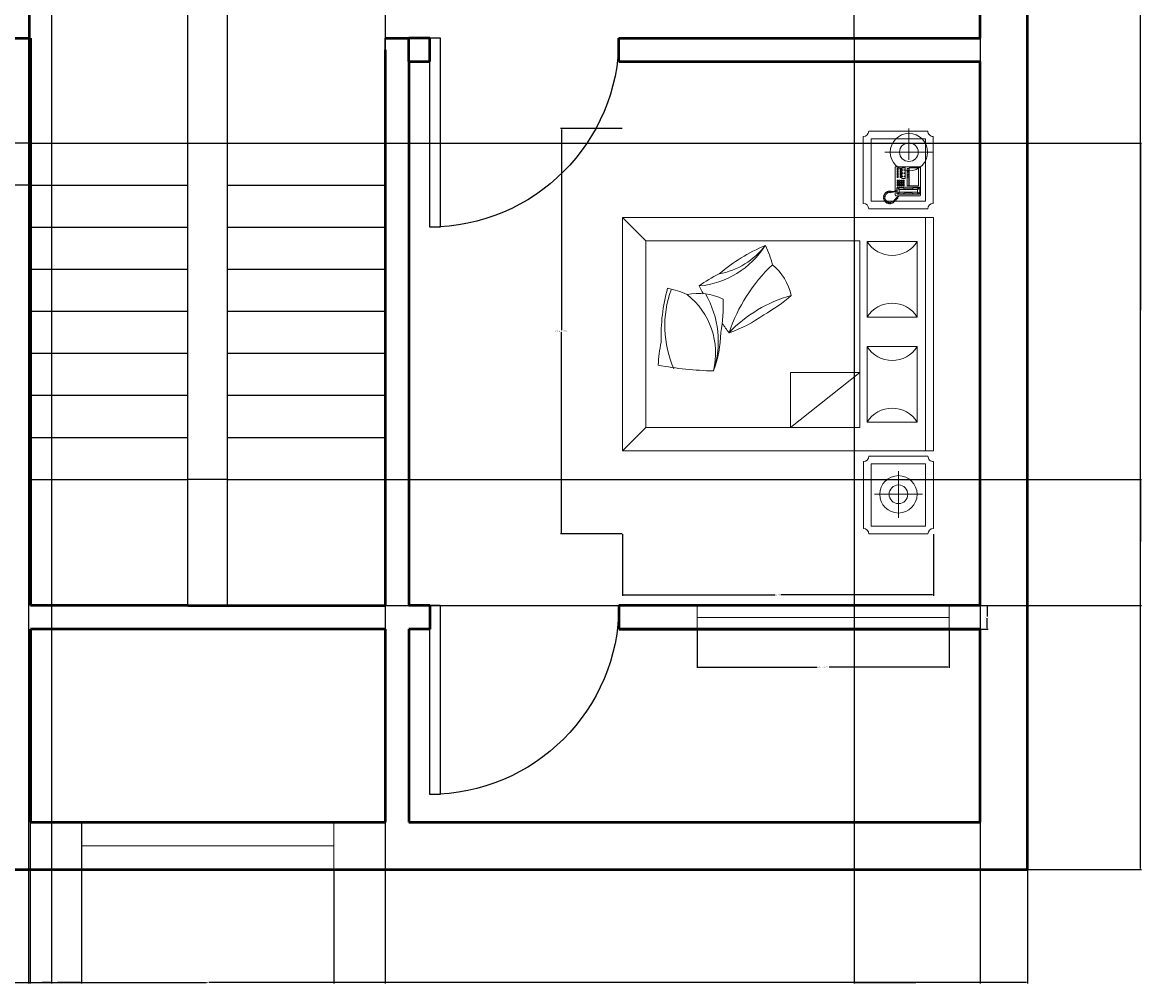
# Model space of a CAD drawing. Units: inches. Extents: x -108 to 1456, y -102 to 617.
# Tile 3 of 8: x 347 to 560, y 154 to 337. Entities that reach past the tile are written whole.
import ezdxf

# ---------------------------------------------------------------- set-up
doc = ezdxf.new("R2010")
doc.units = ezdxf.units.IN
for name, color, linetype, lineweight in [('A-ANNO-DIMS', 2, 'Continuous', 18), ('A-DOOR', 3, 'Continuous', 25), ('A-FLOR-CASE', 32, 'Continuous', 25), ('A-FLOR-STRS', 2, 'Continuous', 25), ('A-FURN', 8, 'Continuous', 18), ('A-GLAZ', 4, 'Continuous', 18), ('A-WALL', 7, 'Continuous', 50)]:
    doc.layers.add(name, color=color, linetype=linetype, lineweight=lineweight)
doc.styles.get("Standard").update_dxf_attribs({"font": 'arial.ttf'})
doc.dimstyles.get("Standard").update_dxf_attribs({"dimtxt": 0.18, "dimasz": 0.18, "dimexe": 0.18, "dimexo": 0.0625, "dimgap": 0.09, "dimtad": 0, "dimtih": 1, "dimtoh": 1, "dimdec": 4, "dimzin": 0, "dimdsep": 46, "dimtxsty": 'Standard', "dimcen": 0.09, "dimadec": 0, "dimazin": 0, "dimtfac": 1, "dimtdec": 4, "dimtofl": 0, "dimtmove": 0, "dimatfit": 3, "dimfxl": 1, "dimtolj": 1, "dimtzin": 0, "dimarcsym": 0})

# ---------------------------------------------------------------- blocks, each defined once
blk = doc.blocks.new('A$C50B66110')
for p, q in [((0.0153, 1.9631), (0.0153, 1.5831)), ((0.0503, 1.9981), (0.4803, 1.9981)), ((0.0653, 1.9481), (0.0653, 1.5981)), ((0.0653, 1.9481), (0.4653, 1.9481)), ((0.1513, 1.6871), (0.1513, 1.9967)), ((0.4653, 1.9481), (0.4653, 1.5981)), ((0.5153, 1.9631), (0.5153, 1.5831)), ((0.5716, 1.9488), (0.5716, 2)), ((0.5716, 2), (2.0719, 2)), ((2.0719, 1.9488), (0.5716, 1.9488)), ((0.5716, 1.9488), (0.5716, 0)), ((2.0719, 1.9488), (2.0719, 2)), ((2.0719, 0), (2.0719, 1.9488)), ((2.1051, 1.9643), (2.1051, 1.5843)), ((2.5701, 1.9993), (2.1401, 1.9993)), ((2.1551, 1.9493), (2.1551, 1.5993)), ((2.5551, 1.9493), (2.1551, 1.9493)), ((2.5551, 1.9493), (2.5551, 1.5993)), ((2.6051, 1.9643), (2.6051, 1.5843)), ((0.7257, 1.5725), (0.7257, 1.8954)), ((0.7257, 1.8954), (1.2113, 1.8954)), ((1.2113, 1.8954), (1.2113, 1.5725)), ((1.4007, 1.5725), (1.4007, 1.8954)), ((1.4007, 1.8954), (1.8863, 1.8954)), ((1.8863, 1.8954), (1.8863, 1.5725)), ((2.3505, 1.62), (2.3505, 1.9295)), ((0, 1.8416), (0.2001, 1.8416)), ((2.5018, 1.7744), (2.2017, 1.7744)), ((0.0653, 1.5981), (0.4653, 1.5981)), ((2.5551, 1.5993), (2.1551, 1.5993)), ((0.0503, 1.5481), (0.4803, 1.5481)), ((1.2113, 1.5725), (0.7257, 1.5725)), ((1.8863, 1.5725), (1.4007, 1.5725)), ((1.5665, 1.5254), (1.5665, 1.0802)), ((1.5665, 1.5254), (1.9219, 1.0802)), ((2.5701, 1.5493), (2.1401, 1.5493)), ((1.9219, 1.0802), (1.5665, 1.0802)), ((0.5716, 0), (0.7216, 0.15)), ((2.0719, 0), (1.9219, 0.15)), ((0.5716, 0), (2.0719, 0))]:
    blk.add_line(p, q)
at = {"linetype": 'ByBlock'}
for p, q in [((0.2481, 1.9162), (0.2458, 1.9139)), ((0.2458, 1.9139), (0.2458, 1.7562)), ((0.2481, 1.9162), (0.4287, 1.9162)), ((0.2526, 1.9036), (0.2526, 1.8431)), ((0.3669, 1.9036), (0.2526, 1.9036)), ((0.3669, 1.8431), (0.3669, 1.9036)), ((0.3772, 1.9071), (0.3818, 1.9128)), ((0.3772, 1.7688), (0.3772, 1.9071)), ((0.3818, 1.9094), (0.3807, 1.9048)), ((0.3807, 1.9048), (0.3807, 1.8739)), ((0.3807, 1.9048), (0.3909, 1.8945)), ((0.3807, 1.8739), (0.3829, 1.8682)), ((0.3818, 1.9128), (0.4161, 1.9128)), ((0.3864, 1.9116), (0.3818, 1.9094)), ((0.3921, 1.8968), (0.3864, 1.9116)), ((0.3864, 1.9116), (0.4138, 1.9116)), ((0.3909, 1.8945), (0.3921, 1.8968)), ((0.3909, 1.8431), (0.3909, 1.8945)), ((0.4081, 1.8968), (0.3921, 1.8968)), ((0.4081, 1.8968), (0.4138, 1.9116)), ((0.4092, 1.8945), (0.4081, 1.8968)), ((0.4195, 1.9048), (0.4092, 1.8945)), ((0.4092, 1.8431), (0.4092, 1.8945)), ((0.4138, 1.9116), (0.4184, 1.9094)), ((0.4161, 1.9128), (0.4218, 1.9071)), ((0.4195, 1.8739), (0.4172, 1.8682)), ((0.4184, 1.9094), (0.4195, 1.9048)), ((0.4195, 1.9048), (0.4195, 1.8739)), ((0.4218, 1.9071), (0.4218, 1.7699)), ((0.4287, 1.9162), (0.4309, 1.9139)), ((0.4309, 1.9139), (0.4309, 1.7562)), ((0.2526, 1.8431), (0.3669, 1.8431)), ((0.3201, 1.8168), (0.2526, 1.8168)), ((0.2526, 1.8168), (0.2526, 1.7962)), ((0.2572, 1.8408), (0.2572, 1.8294)), ((0.3669, 1.8408), (0.2572, 1.8408)), ((0.2572, 1.8294), (0.3669, 1.8294)), ((0.2675, 1.8145), (0.2641, 1.8145)), ((0.2641, 1.8145), (0.2641, 1.8111)), ((0.2641, 1.8111), (0.2675, 1.8111)), ((0.2641, 1.8019), (0.2641, 1.7985)), ((0.2675, 1.8019), (0.2641, 1.8019)), ((0.2641, 1.7985), (0.2675, 1.7985)), ((0.2664, 1.8408), (0.2664, 1.8294)), ((0.2675, 1.8111), (0.2675, 1.8145)), ((0.2675, 1.7985), (0.2675, 1.8019)), ((0.2755, 1.8408), (0.2755, 1.8294)), ((0.2846, 1.8408), (0.2846, 1.8294)), ((0.2846, 1.8145), (0.2846, 1.8111)), ((0.2881, 1.8145), (0.2846, 1.8145)), ((0.2846, 1.8111), (0.2881, 1.8111)), ((0.2846, 1.8019), (0.2846, 1.7985)), ((0.2881, 1.8019), (0.2846, 1.8019)), ((0.2846, 1.7985), (0.2881, 1.7985)), ((0.2881, 1.8111), (0.2881, 1.8145)), ((0.2881, 1.7985), (0.2881, 1.8019)), ((0.2938, 1.8408), (0.2938, 1.8294)), ((0.3029, 1.8408), (0.3029, 1.8294)), ((0.3052, 1.8145), (0.3052, 1.8111)), ((0.3086, 1.8145), (0.3052, 1.8145)), ((0.3052, 1.8111), (0.3086, 1.8111)), ((0.3052, 1.8019), (0.3052, 1.7985)), ((0.3086, 1.8019), (0.3052, 1.8019)), ((0.3052, 1.7985), (0.3086, 1.7985)), ((0.3086, 1.8111), (0.3086, 1.8145)), ((0.3086, 1.7985), (0.3086, 1.8019)), ((0.3121, 1.8408), (0.3121, 1.8294)), ((0.3201, 1.7962), (0.3201, 1.8168)), ((0.3304, 1.8111), (0.3395, 1.8111)), ((0.3304, 1.8042), (0.3304, 1.8111)), ((0.3395, 1.8042), (0.3304, 1.8042)), ((0.3304, 1.7985), (0.3395, 1.7985)), ((0.3304, 1.7916), (0.3304, 1.7985)), ((0.3395, 1.8111), (0.3395, 1.8042)), ((0.3395, 1.7985), (0.3395, 1.7916)), ((0.3441, 1.8042), (0.3441, 1.8111)), ((0.3441, 1.8111), (0.3532, 1.8111)), ((0.3532, 1.8042), (0.3441, 1.8042)), ((0.3441, 1.7985), (0.3532, 1.7985)), ((0.3441, 1.7916), (0.3441, 1.7985)), ((0.3532, 1.8111), (0.3532, 1.8042)), ((0.3532, 1.7985), (0.3532, 1.7916)), ((0.3578, 1.8111), (0.3669, 1.8111)), ((0.3578, 1.8042), (0.3578, 1.8111)), ((0.3669, 1.8042), (0.3578, 1.8042)), ((0.3578, 1.7985), (0.3669, 1.7985)), ((0.3578, 1.7916), (0.3578, 1.7985)), ((0.3669, 1.8294), (0.3669, 1.8408)), ((0.3669, 1.8111), (0.3669, 1.8042)), ((0.3669, 1.7985), (0.3669, 1.7916)), ((0.3807, 1.8019), (0.3829, 1.8076)), ((0.3807, 1.7711), (0.3807, 1.8019)), ((0.3829, 1.8682), (0.3864, 1.8625)), ((0.3829, 1.8076), (0.3864, 1.8134)), ((0.3864, 1.8625), (0.3875, 1.8545)), ((0.3864, 1.8134), (0.3875, 1.8214)), ((0.3875, 1.8545), (0.3875, 1.8431)), ((0.3875, 1.8214), (0.3875, 1.8431)), ((0.3909, 1.8431), (0.3909, 1.7813)), ((0.4092, 1.8431), (0.4092, 1.7813)), ((0.4138, 1.8625), (0.4127, 1.8545)), ((0.4127, 1.8545), (0.4127, 1.8431)), ((0.4127, 1.8214), (0.4127, 1.8431)), ((0.4138, 1.8134), (0.4127, 1.8214)), ((0.4172, 1.8682), (0.4138, 1.8625)), ((0.4172, 1.8076), (0.4138, 1.8134)), ((0.4195, 1.8019), (0.4172, 1.8076)), ((0.4195, 1.7711), (0.4195, 1.8019)), ((0.2458, 1.7562), (0.2481, 1.7539)), ((0.4, 1.7539), (0.2481, 1.7539)), ((0.2526, 1.7962), (0.3201, 1.7962)), ((0.2652, 1.7905), (0.2538, 1.7905)), ((0.2538, 1.7905), (0.2538, 1.7859)), ((0.2538, 1.7859), (0.2652, 1.7859)), ((0.2538, 1.7665), (0.2538, 1.7733)), ((0.2538, 1.7733), (0.2652, 1.7733)), ((0.2652, 1.7665), (0.2538, 1.7665)), ((0.2652, 1.7859), (0.2652, 1.7905)), ((0.2652, 1.7733), (0.2652, 1.7665)), ((0.2812, 1.7905), (0.2698, 1.7905)), ((0.2698, 1.7905), (0.2698, 1.7859)), ((0.2698, 1.7859), (0.2812, 1.7859)), ((0.2698, 1.7665), (0.2698, 1.7733)), ((0.2698, 1.7733), (0.2812, 1.7733)), ((0.2812, 1.7665), (0.2698, 1.7665)), ((0.2812, 1.7859), (0.2812, 1.7905)), ((0.2812, 1.7733), (0.2812, 1.7665)), ((0.2972, 1.7905), (0.2858, 1.7905)), ((0.2858, 1.7905), (0.2858, 1.7859)), ((0.2858, 1.7859), (0.2972, 1.7859)), ((0.2858, 1.7665), (0.2858, 1.7733)), ((0.2858, 1.7733), (0.2972, 1.7733)), ((0.2972, 1.7665), (0.2858, 1.7665)), ((0.2972, 1.7859), (0.2972, 1.7905)), ((0.2972, 1.7733), (0.2972, 1.7665)), ((0.3018, 1.7905), (0.3018, 1.7859)), ((0.3132, 1.7905), (0.3018, 1.7905)), ((0.3018, 1.7859), (0.3132, 1.7859)), ((0.3018, 1.7733), (0.3132, 1.7733)), ((0.3018, 1.7665), (0.3018, 1.7733)), ((0.3132, 1.7665), (0.3018, 1.7665)), ((0.3132, 1.7859), (0.3132, 1.7905)), ((0.3132, 1.7733), (0.3132, 1.7665)), ((0.3395, 1.7916), (0.3304, 1.7916)), ((0.3304, 1.7779), (0.3304, 1.7848)), ((0.3304, 1.7848), (0.3395, 1.7848)), ((0.3395, 1.7779), (0.3304, 1.7779)), ((0.3304, 1.7722), (0.3395, 1.7722)), ((0.3304, 1.7653), (0.3304, 1.7722)), ((0.3395, 1.7653), (0.3304, 1.7653)), ((0.3395, 1.7848), (0.3395, 1.7779)), ((0.3395, 1.7722), (0.3395, 1.7653)), ((0.3532, 1.7916), (0.3441, 1.7916)), ((0.3441, 1.7779), (0.3441, 1.7848)), ((0.3441, 1.7848), (0.3532, 1.7848)), ((0.3532, 1.7779), (0.3441, 1.7779)), ((0.3441, 1.7722), (0.3532, 1.7722)), ((0.3441, 1.7653), (0.3441, 1.7722)), ((0.3532, 1.7653), (0.3441, 1.7653)), ((0.3532, 1.7848), (0.3532, 1.7779)), ((0.3532, 1.7722), (0.3532, 1.7653)), ((0.3669, 1.7916), (0.3578, 1.7916)), ((0.3578, 1.7791), (0.3578, 1.7859)), ((0.3578, 1.7859), (0.3669, 1.7859)), ((0.3669, 1.7791), (0.3578, 1.7791)), ((0.3578, 1.7653), (0.3578, 1.7722)), ((0.3578, 1.7722), (0.3669, 1.7722)), ((0.3669, 1.7653), (0.3578, 1.7653)), ((0.3669, 1.7859), (0.3669, 1.7791)), ((0.3669, 1.7722), (0.3669, 1.7653)), ((0.3829, 1.7631), (0.3772, 1.7688)), ((0.3807, 1.7711), (0.3909, 1.7813)), ((0.3818, 1.7665), (0.3807, 1.7711)), ((0.3864, 1.7642), (0.3818, 1.7665)), ((0.399, 1.7631), (0.3829, 1.7631)), ((0.3921, 1.7791), (0.3864, 1.7642)), ((0.3864, 1.7642), (0.399, 1.7642)), ((0.3909, 1.7813), (0.3921, 1.7791)), ((0.4081, 1.7791), (0.3921, 1.7791)), ((0.4024, 1.7676), (0.3989, 1.7676)), ((0.3989, 1.7676), (0.3991, 1.7578)), ((0.3991, 1.7578), (0.4019, 1.7462)), ((0.4019, 1.7462), (0.4047, 1.7353)), ((0.403, 1.7585), (0.4024, 1.7676)), ((0.4026, 1.7642), (0.4138, 1.7642)), ((0.4051, 1.7279), (0.4026, 1.7254)), ((0.4161, 1.7631), (0.4027, 1.7631)), ((0.4047, 1.7511), (0.403, 1.7585)), ((0.4287, 1.7539), (0.404, 1.7539)), ((0.4047, 1.7353), (0.4044, 1.7293)), ((0.4044, 1.7293), (0.4051, 1.7279)), ((0.4074, 1.7402), (0.4047, 1.7511)), ((0.4081, 1.7346), (0.4074, 1.7402)), ((0.4079, 1.7286), (0.4081, 1.7346)), ((0.4121, 1.7256), (0.4079, 1.7286)), ((0.4092, 1.7813), (0.4081, 1.7791)), ((0.4081, 1.7791), (0.4138, 1.7642)), ((0.4195, 1.7711), (0.4092, 1.7813)), ((0.4138, 1.7642), (0.4184, 1.7665)), ((0.4218, 1.7699), (0.4161, 1.7631)), ((0.4184, 1.7665), (0.4195, 1.7711)), ((0.4309, 1.7562), (0.4287, 1.7539)), ((0.4378, 1.7742), (0.4309, 1.7768)), ((0.4309, 1.7722), (0.436, 1.7708)), ((0.436, 1.7708), (0.4406, 1.7672)), ((0.441, 1.771), (0.4378, 1.7742)), ((0.4406, 1.7672), (0.4418, 1.7656)), ((0.4434, 1.7688), (0.441, 1.771)), ((0.4443, 1.7658), (0.4418, 1.7633)), ((0.4418, 1.7656), (0.4443, 1.7658)), ((0.4418, 1.7633), (0.4511, 1.7551)), ((0.4477, 1.7704), (0.4434, 1.7688)), ((0.4497, 1.7684), (0.4477, 1.7704)), ((0.4481, 1.765), (0.4497, 1.7684)), ((0.4509, 1.7672), (0.4481, 1.765)), ((0.4539, 1.764), (0.4509, 1.7672)), ((0.4511, 1.7551), (0.4662, 1.7422)), ((0.4515, 1.7573), (0.4539, 1.764)), ((0.4577, 1.7605), (0.4515, 1.7573)), ((0.463, 1.7555), (0.4577, 1.7605)), ((0.4618, 1.7482), (0.463, 1.7555)), ((0.467, 1.7515), (0.4618, 1.7482)), ((0.4664, 1.7418), (0.4741, 1.72)), ((0.4714, 1.7468), (0.467, 1.7515)), ((0.4696, 1.7418), (0.4714, 1.7468)), ((0.4766, 1.7425), (0.4697, 1.7418)), ((0.472, 1.733), (0.4787, 1.7356)), ((0.4794, 1.7332), (0.472, 1.733)), ((0.4761, 1.7233), (0.481, 1.7279)), ((0.4787, 1.7356), (0.4766, 1.7425)), ((0.481, 1.7279), (0.4794, 1.7332)), ((0.4026, 1.7254), (0.4021, 1.7198)), ((0.4021, 1.7198), (0.4088, 1.7187)), ((0.4088, 1.7187), (0.4023, 1.7147)), ((0.4023, 1.7147), (0.4028, 1.7085)), ((0.4028, 1.7085), (0.4102, 1.7078)), ((0.4102, 1.7078), (0.4037, 1.7027)), ((0.4037, 1.7027), (0.4067, 1.6974)), ((0.4067, 1.6974), (0.4137, 1.6988)), ((0.4137, 1.6988), (0.4104, 1.6923)), ((0.4104, 1.6923), (0.4139, 1.6881)), ((0.4111, 1.7203), (0.4121, 1.7256)), ((0.4123, 1.7057), (0.4111, 1.7203)), ((0.4211, 1.6946), (0.4123, 1.7057)), ((0.4139, 1.6881), (0.4192, 1.692)), ((0.4192, 1.692), (0.4183, 1.6858)), ((0.4183, 1.6858), (0.4227, 1.683)), ((0.4333, 1.6881), (0.4211, 1.6946)), ((0.4227, 1.683), (0.4283, 1.6876)), ((0.4283, 1.6876), (0.4276, 1.68)), ((0.4276, 1.68), (0.4324, 1.6786)), ((0.4324, 1.6786), (0.4354, 1.6849)), ((0.4472, 1.6869), (0.4333, 1.6881)), ((0.4354, 1.6849), (0.4382, 1.6786)), ((0.4382, 1.6786), (0.4421, 1.6782)), ((0.4421, 1.6782), (0.4437, 1.6849)), ((0.4437, 1.6849), (0.4463, 1.6775)), ((0.4463, 1.6775), (0.4507, 1.6786)), ((0.4606, 1.6927), (0.4472, 1.6869)), ((0.4507, 1.6786), (0.4509, 1.6849)), ((0.4509, 1.6849), (0.4562, 1.6802)), ((0.4562, 1.6802), (0.4599, 1.6821)), ((0.4592, 1.689), (0.4641, 1.683)), ((0.4599, 1.6821), (0.4592, 1.689)), ((0.4708, 1.7027), (0.4606, 1.6927)), ((0.4641, 1.683), (0.4678, 1.6863)), ((0.465, 1.6925), (0.4715, 1.6897)), ((0.4678, 1.6863), (0.465, 1.6925)), ((0.4741, 1.72), (0.4708, 1.7027)), ((0.4745, 1.6925), (0.4713, 1.6988)), ((0.4713, 1.6988), (0.478, 1.6967)), ((0.4715, 1.6897), (0.4745, 1.6925)), ((0.4743, 1.7075), (0.4815, 1.7073)), ((0.4798, 1.7013), (0.4743, 1.7075)), ((0.4824, 1.7233), (0.4761, 1.7233)), ((0.4764, 1.7154), (0.4835, 1.7175)), ((0.4824, 1.7119), (0.4764, 1.7154)), ((0.478, 1.6967), (0.4798, 1.7013)), ((0.4815, 1.7073), (0.4824, 1.7119)), ((0.4835, 1.7175), (0.4824, 1.7233)), ((0.7216, 1.5254), (1.9219, 1.5254)), ((0.7216, 1.5254), (0.7216, 0.15)), ((1.9219, 0.15), (1.9219, 1.5254)), ((0.7216, 0.15), (1.9219, 0.15))]:
    blk.add_line(p, q, dxfattribs=at)
for centre, radius in [((0.1513, 1.8416), 0.12), ((0.1513, 1.8416), 0.06), ((2.3505, 1.7744), 0.12), ((2.3505, 1.7744), 0.06)]:
    blk.add_circle(centre, radius)
for centre, radius, start, end in [((0.0153, 1.9981), 0.035, 270, 0), ((0.5153, 1.9981), 0.035, 180, 270), ((2.1051, 1.9993), 0.035, 270, 0), ((2.6051, 1.9993), 0.035, 180, 270), ((0.6244, 1.734), 0.1906, 302.12017, 57.87983), ((1.3126, 1.734), 0.1906, 122.12017, 237.87983), ((1.2994, 1.734), 0.1906, 302.12017, 57.87983), ((1.9876, 1.734), 0.1906, 122.12017, 237.87983), ((0.0153, 1.5481), 0.035, 0, 90), ((0.5153, 1.5481), 0.035, 90, 180), ((2.1051, 1.5493), 0.035, 0, 90), ((2.6051, 1.5493), 0.035, 90, 180), ((1.1502, 0.7366), 0.3575, 102.47819, 140.46254), ((0.328, 0.4368), 0.9879, 28.49711, 41.05657), ((1.9117, 1.3157), 0.8697, 195.33601, 226.41927), ((0.9996, 0.4307), 0.548, 103.20343, 117.03623), ((1.656, 1.7093), 1.0798, 223.63057, 251.4288), ((0.4482, 0.4408), 0.5655, 5.33912, 57.68949), ((1.8226, 1.3753), 1.1652, 203.06416, 220.32086), ((0.4548, 0.5307), 0.4879, 10.69865, 52.68638), ((0.5648, 0.4378), 0.7874, 18.35266, 36.68512), ((1.1403, -0.3401), 0.9879, 80.06073, 92.62018), ((-0.0179, 2.4352), 2.1977, 305.29657, 307.24182), ((1.5981, 0.9345), 0.734, 205.25901, 216.93514), ((1.4166, 0.4903), 0.3575, 154.0418, 192.02615), ((1.3672, 0.0075), 0.6085, 71.81005, 120.13512), ((1.4431, 0.1219), 0.4774, 76.18494, 142.00166), ((1.2867, -0.154), 0.7874, 69.91627, 88.24873), ((-0.6401, 0.6314), 2.1977, 349.48843, 358.80544), ((-0.0179, 2.4352), 2.1977, 297.92482, 299.3793), ((1.5626, 0.1822), 0.548, 154.76704, 168.59984), ((1.3343, 1.4141), 1.1652, 254.62778, 271.88448), ((1.2678, 0.9611), 0.6885, 250.29361, 293.6414), ((1.5399, 0.9642), 0.734, 256.82263, 268.49876)]:
    blk.add_arc(centre, radius, start, end)
blk = doc.blocks.new('DOOR-36-SWING')
for p, q in [((36, 36), (34, 36)), ((34, 36), (34, 0)), ((36, 36), (34, 36)), ((36, 0), (36, 36)), ((34, 0), (36, 0))]:
    blk.add_line(p, q)
blk.add_arc((36, 36), 36, 180, 270)
blk = doc.blocks.new('WIN-48-WALL-4_5')
for p, q in [((0, 0), (0, 4.5)), ((48, 0), (48, 4.5)), ((0, 2.25), (48, 2.25))]:
    blk.add_line(p, q)
blk = doc.blocks.new('*D18')
at = {"layer": 'A-ANNO-DIMS', "color": 0, "lineweight": -2, "transparency": 16777216}
for p, q in [((475.47, 221.46), (475.47, 214.14)), ((523.47, 221.46), (523.47, 214.14)), ((475.65, 214.32), (498.35, 214.32)), ((523.29, 214.32), (500.59, 214.32))]:
    blk.add_line(p, q, dxfattribs=at)
at = {"layer": 'A-ANNO-DIMS', "color": 0, "transparency": 16777216}
for points in [[(475.65, 214.35), (475.65, 214.29), (475.47, 214.32)], [(523.29, 214.35), (523.29, 214.29), (523.47, 214.32)]]:
    blk.add_solid(points, dxfattribs=at)
at = {"layer": 'Defpoints', "color": 0, "transparency": 16777216}
for p in [(475.47, 221.52), (523.47, 221.52), (523.47, 214.32)]:
    blk.add_point(p, dxfattribs=at)
at = {"layer": 'A-ANNO-DIMS', "color": 0, "transparency": 16777216, "insert": (499.47, 214.32), "char_height": 0.18, "attachment_point": 5}
blk.add_mtext('\\A1;WINDOW 48 TYP.', dxfattribs=at)
blk = doc.blocks.new('*D19')
at = {"layer": 'A-ANNO-DIMS', "color": 0, "lineweight": -2, "transparency": 16777216}
for p, q in [((523.53, 226.02), (530.85, 226.02)), ((530.67, 225.84), (530.67, 223.96)), ((523.53, 221.52), (530.85, 221.52)), ((530.67, 221.7), (530.67, 223.59))]:
    blk.add_line(p, q, dxfattribs=at)
at = {"layer": 'A-ANNO-DIMS', "color": 0, "transparency": 16777216}
for points in [[(530.64, 225.84), (530.7, 225.84), (530.67, 226.02)], [(530.64, 221.7), (530.7, 221.7), (530.67, 221.52)]]:
    blk.add_solid(points, dxfattribs=at)
at = {"layer": 'Defpoints', "color": 0, "transparency": 16777216}
for p in [(523.47, 226.02), (530.67, 226.02), (523.47, 221.52)]:
    blk.add_point(p, dxfattribs=at)
at = {"layer": 'A-ANNO-DIMS', "color": 0, "transparency": 16777216, "insert": (530.67, 223.77), "char_height": 0.18, "attachment_point": 5}
blk.add_mtext('\\A1;5 TYP.', dxfattribs=at)
blk = doc.blocks.new('*D22')
at = {"layer": 'A-ANNO-DIMS', "color": 0, "lineweight": -2, "transparency": 16777216}
for p, q in [((461.2, 316.78), (449.51, 316.78)), ((449.69, 316.6), (449.69, 278.4)), ((449.69, 239.82), (449.69, 278.03)), ((461.2, 239.64), (449.51, 239.64))]:
    blk.add_line(p, q, dxfattribs=at)
at = {"layer": 'A-ANNO-DIMS', "color": 0, "transparency": 16777216}
for points in [[(449.66, 316.6), (449.72, 316.6), (449.69, 316.78)], [(449.66, 239.82), (449.72, 239.82), (449.69, 239.64)]]:
    blk.add_solid(points, dxfattribs=at)
at = {"layer": 'Defpoints', "color": 0, "transparency": 16777216}
for p in [(461.26, 316.78), (449.69, 239.64), (461.26, 239.64)]:
    blk.add_point(p, dxfattribs=at)
at = {"layer": 'A-ANNO-DIMS', "color": 0, "transparency": 16777216, "insert": (449.69, 278.21), "char_height": 0.18, "attachment_point": 5}
blk.add_mtext('\\A1;BED GROUP 77 TYP.', dxfattribs=at)
blk = doc.blocks.new('*D23')
at = {"layer": 'A-ANNO-DIMS', "color": 0, "lineweight": -2, "transparency": 16777216}
for p, q in [((461.26, 239.58), (461.26, 227.89)), ((520.48, 239.58), (520.48, 227.89)), ((461.44, 228.07), (490.34, 228.07)), ((520.3, 228.07), (491.4, 228.07))]:
    blk.add_line(p, q, dxfattribs=at)
at = {"layer": 'A-ANNO-DIMS', "color": 0, "transparency": 16777216}
for points in [[(461.44, 228.1), (461.44, 228.04), (461.26, 228.07)], [(520.3, 228.1), (520.3, 228.04), (520.48, 228.07)]]:
    blk.add_solid(points, dxfattribs=at)
at = {"layer": 'Defpoints', "color": 0, "transparency": 16777216}
for p in [(461.26, 239.64), (520.48, 239.64), (520.48, 228.07)]:
    blk.add_point(p, dxfattribs=at)
at = {"layer": 'A-ANNO-DIMS', "color": 0, "transparency": 16777216, "insert": (490.87, 228.07), "char_height": 0.18, "attachment_point": 5}
blk.add_mtext('\\A1;59 TYP.', dxfattribs=at)
blk = doc.blocks.new('*D34')
at = {"layer": 'A-ANNO-DIMS', "color": 0, "lineweight": -2, "transparency": 16777216}
for p, q in [((226.34, 175.71), (226.34, 154.07)), ((538.34, 175.71), (538.34, 154.07)), ((226.52, 154.25), (382.06, 154.25)), ((538.16, 154.25), (382.63, 154.25))]:
    blk.add_line(p, q, dxfattribs=at)
at = {"layer": 'A-ANNO-DIMS', "color": 0, "transparency": 16777216}
for points in [[(226.52, 154.28), (226.52, 154.22), (226.34, 154.25)], [(538.16, 154.28), (538.16, 154.22), (538.34, 154.25)]]:
    blk.add_solid(points, dxfattribs=at)
at = {"layer": 'Defpoints', "color": 0, "transparency": 16777216}
for p in [(226.34, 175.77), (538.34, 175.77), (538.34, 154.25)]:
    blk.add_point(p, dxfattribs=at)
at = {"layer": 'A-ANNO-DIMS', "color": 0, "transparency": 16777216, "insert": (382.34, 154.25), "char_height": 0.18, "attachment_point": 5}
blk.add_mtext('\\A1;312', dxfattribs=at)
blk = doc.blocks.new('*D35')
at = {"layer": 'A-ANNO-DIMS', "color": 0, "lineweight": -2, "transparency": 16777216}
for p, q in [((538.41, 595.77), (560.05, 595.77)), ((559.87, 595.59), (559.87, 385.96)), ((559.87, 175.95), (559.87, 385.59)), ((538.41, 175.77), (560.05, 175.77))]:
    blk.add_line(p, q, dxfattribs=at)
at = {"layer": 'A-ANNO-DIMS', "color": 0, "transparency": 16777216}
for points in [[(559.84, 595.59), (559.9, 595.59), (559.87, 595.77)], [(559.84, 175.95), (559.9, 175.95), (559.87, 175.77)]]:
    blk.add_solid(points, dxfattribs=at)
at = {"layer": 'Defpoints', "color": 0, "transparency": 16777216}
for p in [(538.34, 595.77), (559.87, 595.77), (538.34, 175.77)]:
    blk.add_point(p, dxfattribs=at)
at = {"layer": 'A-ANNO-DIMS', "color": 0, "transparency": 16777216, "insert": (559.87, 385.77), "char_height": 0.18, "attachment_point": 5}
blk.add_mtext('\\A1;420', dxfattribs=at)
blk = doc.blocks.new('*D49')
at = {"layer": 'A-ANNO-DIMS', "color": 0, "lineweight": -2, "transparency": 16777216}
for p, q in [((348.27, 521.46), (348.27, 154.07)), ((416.09, 521.46), (416.09, 154.07)), ((348.45, 154.25), (381.79, 154.25)), ((415.91, 154.25), (382.57, 154.25))]:
    blk.add_line(p, q, dxfattribs=at)
at = {"layer": 'A-ANNO-DIMS', "color": 0, "transparency": 16777216}
for points in [[(348.45, 154.28), (348.45, 154.22), (348.27, 154.25)], [(415.91, 154.28), (415.91, 154.22), (416.09, 154.25)]]:
    blk.add_solid(points, dxfattribs=at)
at = {"layer": 'Defpoints', "color": 0, "transparency": 16777216}
for p in [(348.27, 521.52), (416.09, 521.52), (416.09, 154.25)]:
    blk.add_point(p, dxfattribs=at)
at = {"layer": 'A-ANNO-DIMS', "color": 0, "transparency": 16777216, "insert": (382.18, 154.25), "char_height": 0.18, "attachment_point": 5}
blk.add_mtext('\\A1;67.83', dxfattribs=at)
blk = doc.blocks.new('*D53')
at = {"layer": 'A-ANNO-DIMS', "color": 0, "lineweight": -2, "transparency": 16777216}
for p, q in [((348.27, 453.96), (348.27, 154.07)), ((352.59, 453.96), (352.59, 154.07)), ((348.45, 154.25), (350.03, 154.25)), ((352.41, 154.25), (350.83, 154.25))]:
    blk.add_line(p, q, dxfattribs=at)
at = {"layer": 'A-ANNO-DIMS', "color": 0, "transparency": 16777216}
for points in [[(348.45, 154.28), (348.45, 154.22), (348.27, 154.25)], [(352.41, 154.28), (352.41, 154.22), (352.59, 154.25)]]:
    blk.add_solid(points, dxfattribs=at)
at = {"layer": 'Defpoints', "color": 0, "transparency": 16777216}
for p in [(348.27, 454.02), (352.59, 454.02), (352.59, 154.25)]:
    blk.add_point(p, dxfattribs=at)
at = {"layer": 'A-ANNO-DIMS', "color": 0, "transparency": 16777216, "insert": (350.43, 154.25), "char_height": 0.18, "attachment_point": 5}
blk.add_mtext('\\A1;4.328', dxfattribs=at)
blk = doc.blocks.new('*D55')
at = {"layer": 'A-ANNO-DIMS', "color": 0, "lineweight": -2, "transparency": 16777216}
for p, q in [((358.34, 175.71), (358.34, 154.07)), ((406.34, 175.71), (406.34, 154.07)), ((358.52, 154.25), (382.12, 154.25)), ((406.16, 154.25), (382.57, 154.25))]:
    blk.add_line(p, q, dxfattribs=at)
at = {"layer": 'A-ANNO-DIMS', "color": 0, "transparency": 16777216}
for points in [[(358.52, 154.28), (358.52, 154.22), (358.34, 154.25)], [(406.16, 154.28), (406.16, 154.22), (406.34, 154.25)]]:
    blk.add_solid(points, dxfattribs=at)
at = {"layer": 'Defpoints', "color": 0, "transparency": 16777216}
for p in [(358.34, 175.77), (406.34, 175.77), (406.34, 154.25)]:
    blk.add_point(p, dxfattribs=at)
at = {"layer": 'A-ANNO-DIMS', "color": 0, "transparency": 16777216, "insert": (382.34, 154.25), "char_height": 0.18, "attachment_point": 5}
blk.add_mtext('\\A1;48', dxfattribs=at)
blk = doc.blocks.new('*D56')
at = {"layer": 'A-ANNO-DIMS', "color": 0, "lineweight": -2, "transparency": 16777216}
for p, q in [((348.59, 184.71), (348.59, 154.07)), ((358.34, 184.71), (358.34, 154.07)), ((348.77, 154.25), (353.14, 154.25)), ((358.16, 154.25), (353.79, 154.25))]:
    blk.add_line(p, q, dxfattribs=at)
at = {"layer": 'A-ANNO-DIMS', "color": 0, "transparency": 16777216}
for points in [[(348.77, 154.28), (348.77, 154.22), (348.59, 154.25)], [(358.16, 154.28), (358.16, 154.22), (358.34, 154.25)]]:
    blk.add_solid(points, dxfattribs=at)
at = {"layer": 'Defpoints', "color": 0, "transparency": 16777216}
for p in [(348.59, 184.77), (358.34, 184.77), (358.34, 154.25)]:
    blk.add_point(p, dxfattribs=at)
at = {"layer": 'A-ANNO-DIMS', "color": 0, "transparency": 16777216, "insert": (353.47, 154.25), "char_height": 0.18, "attachment_point": 5}
blk.add_mtext('\\A1;9.75', dxfattribs=at)
blk = doc.blocks.new('*D59')
at = {"layer": 'A-ANNO-DIMS', "color": 0, "lineweight": -2, "transparency": 16777216}
for p, q in [((505.34, 333.96), (505.34, 154.07)), ((529.34, 333.96), (529.34, 154.07)), ((505.52, 154.25), (517.12, 154.25)), ((529.16, 154.25), (517.56, 154.25))]:
    blk.add_line(p, q, dxfattribs=at)
at = {"layer": 'A-ANNO-DIMS', "color": 0, "transparency": 16777216}
for points in [[(505.52, 154.28), (505.52, 154.22), (505.34, 154.25)], [(529.16, 154.28), (529.16, 154.22), (529.34, 154.25)]]:
    blk.add_solid(points, dxfattribs=at)
at = {"layer": 'Defpoints', "color": 0, "transparency": 16777216}
for p in [(505.34, 334.02), (529.34, 334.02), (529.34, 154.25)]:
    blk.add_point(p, dxfattribs=at)
at = {"layer": 'A-ANNO-DIMS', "color": 0, "transparency": 16777216, "insert": (517.34, 154.25), "char_height": 0.18, "attachment_point": 5}
blk.add_mtext('\\A1;24', dxfattribs=at)
blk = doc.blocks.new('*D61')
at = {"layer": 'A-ANNO-DIMS', "color": 0, "lineweight": -2, "transparency": 16777216}
for p, q in [((416.16, 314.02), (560.05, 314.02)), ((559.87, 313.84), (559.87, 282.21)), ((559.87, 250.2), (559.87, 281.84)), ((416.16, 250.02), (560.05, 250.02))]:
    blk.add_line(p, q, dxfattribs=at)
at = {"layer": 'A-ANNO-DIMS', "color": 0, "transparency": 16777216}
for points in [[(559.84, 313.84), (559.9, 313.84), (559.87, 314.02)], [(559.84, 250.2), (559.9, 250.2), (559.87, 250.02)]]:
    blk.add_solid(points, dxfattribs=at)
at = {"layer": 'Defpoints', "color": 0, "transparency": 16777216}
for p in [(416.09, 314.02), (416.09, 250.02), (559.87, 250.02)]:
    blk.add_point(p, dxfattribs=at)
at = {"layer": 'A-ANNO-DIMS', "color": 0, "transparency": 16777216, "insert": (559.87, 282.02), "char_height": 0.18, "attachment_point": 5}
blk.add_mtext('\\A1;64', dxfattribs=at)
blk = doc.blocks.new('*D62')
at = {"layer": 'A-ANNO-DIMS', "color": 0, "lineweight": -2, "transparency": 16777216}
for p, q in [((348.59, 314.09), (348.59, 617.48)), ((348.77, 617.3), (363.38, 617.3)), ((378.41, 617.3), (363.81, 617.3)), ((378.59, 314.09), (378.59, 617.48))]:
    blk.add_line(p, q, dxfattribs=at)
at = {"layer": 'A-ANNO-DIMS', "color": 0, "transparency": 16777216}
for points in [[(348.77, 617.33), (348.77, 617.27), (348.59, 617.3)], [(378.41, 617.33), (378.41, 617.27), (378.59, 617.3)]]:
    blk.add_solid(points, dxfattribs=at)
at = {"layer": 'Defpoints', "color": 0, "transparency": 16777216}
for p in [(378.59, 617.3), (348.59, 314.02), (378.59, 314.02)]:
    blk.add_point(p, dxfattribs=at)
at = {"layer": 'A-ANNO-DIMS', "color": 0, "transparency": 16777216, "insert": (363.59, 617.3), "char_height": 0.18, "attachment_point": 5}
blk.add_mtext('\\A1;30', dxfattribs=at)
blk = doc.blocks.new('*D63')
at = {"layer": 'A-ANNO-DIMS', "color": 0, "lineweight": -2, "transparency": 16777216}
for p, q in [((378.59, 314.09), (378.59, 617.48)), ((378.77, 617.3), (382.09, 617.3)), ((385.91, 617.3), (382.6, 617.3)), ((386.09, 314.09), (386.09, 617.48))]:
    blk.add_line(p, q, dxfattribs=at)
at = {"layer": 'A-ANNO-DIMS', "color": 0, "transparency": 16777216}
for points in [[(378.77, 617.33), (378.77, 617.27), (378.59, 617.3)], [(385.91, 617.33), (385.91, 617.27), (386.09, 617.3)]]:
    blk.add_solid(points, dxfattribs=at)
at = {"layer": 'Defpoints', "color": 0, "transparency": 16777216}
for p in [(386.09, 617.3), (378.59, 314.02), (386.09, 314.02)]:
    blk.add_point(p, dxfattribs=at)
at = {"layer": 'A-ANNO-DIMS', "color": 0, "transparency": 16777216, "insert": (382.34, 617.3), "char_height": 0.18, "attachment_point": 5}
blk.add_mtext('\\A1;7.5', dxfattribs=at)
blk = doc.blocks.new('*D64')
at = {"layer": 'A-ANNO-DIMS', "color": 0, "lineweight": -2, "transparency": 16777216}
for p, q in [((348.53, 314.02), (204.64, 314.02)), ((204.82, 313.84), (204.82, 310.21)), ((204.82, 306.2), (204.82, 309.84)), ((348.53, 306.02), (204.64, 306.02))]:
    blk.add_line(p, q, dxfattribs=at)
at = {"layer": 'A-ANNO-DIMS', "color": 0, "transparency": 16777216}
for points in [[(204.79, 313.84), (204.85, 313.84), (204.82, 314.02)], [(204.79, 306.2), (204.85, 306.2), (204.82, 306.02)]]:
    blk.add_solid(points, dxfattribs=at)
at = {"layer": 'Defpoints', "color": 0, "transparency": 16777216}
for p in [(348.59, 314.02), (204.82, 306.02), (348.59, 306.02)]:
    blk.add_point(p, dxfattribs=at)
at = {"layer": 'A-ANNO-DIMS', "color": 0, "transparency": 16777216, "insert": (204.82, 310.02), "char_height": 0.18, "attachment_point": 5}
blk.add_mtext('\\A1;8', dxfattribs=at)
blk = doc.blocks.new('*D65')
at = {"layer": 'A-ANNO-DIMS', "color": 0, "lineweight": -2, "transparency": 16777216}
for p, q in [((416.16, 250.02), (560.05, 250.02)), ((559.87, 249.84), (559.87, 238.2)), ((559.87, 226.2), (559.87, 237.84)), ((416.16, 226.02), (560.05, 226.02))]:
    blk.add_line(p, q, dxfattribs=at)
at = {"layer": 'A-ANNO-DIMS', "color": 0, "transparency": 16777216}
for points in [[(559.84, 249.84), (559.9, 249.84), (559.87, 250.02)], [(559.84, 226.2), (559.9, 226.2), (559.87, 226.02)]]:
    blk.add_solid(points, dxfattribs=at)
at = {"layer": 'Defpoints', "color": 0, "transparency": 16777216}
for p in [(416.09, 250.02), (559.87, 250.02), (416.09, 226.02)]:
    blk.add_point(p, dxfattribs=at)
at = {"layer": 'A-ANNO-DIMS', "color": 0, "transparency": 16777216, "insert": (559.87, 238.02), "char_height": 0.18, "attachment_point": 5}
blk.add_mtext('\\A1;24', dxfattribs=at)

msp = doc.modelspace()

# ---------------------------------------------------------------- linework, layer by layer
at = {"layer": 'A-FLOR-CASE'}
for p, q in [((505.3443, 334.021), (505.3443, 425.5243)), ((529.3443, 334.021), (529.3443, 425.5243))]:
    msp.add_line(p, q, dxfattribs=at)
at = {"layer": 'A-FLOR-STRS'}
for p, q in [((416.0943, 226.0243), (416.0943, 333.995)), ((348.5943, 226.0243), (348.5943, 329.5243)), ((348.5943, 314.0243), (416.0943, 314.0243)), ((378.5943, 226.0243), (378.5943, 314.0243)), ((386.0943, 226.0243), (386.0943, 314.0243)), ((348.5943, 306.0243), (378.5943, 306.0243)), ((348.5943, 306.0243), (378.5943, 306.0243)), ((386.0943, 306.0243), (416.0943, 306.0243)), ((386.0943, 306.0243), (416.0943, 306.0243)), ((348.5943, 298.0243), (378.5943, 298.0243)), ((348.5943, 298.0243), (378.5943, 298.0243)), ((386.0943, 298.0243), (416.0943, 298.0243)), ((386.0943, 298.0243), (416.0943, 298.0243)), ((348.5943, 290.0243), (378.5943, 290.0243)), ((348.5943, 290.0243), (378.5943, 290.0243)), ((386.0943, 290.0243), (416.0943, 290.0243)), ((386.0943, 290.0243), (416.0943, 290.0243)), ((348.5943, 282.0243), (378.5943, 282.0243)), ((348.5943, 282.0243), (378.5943, 282.0243)), ((386.0943, 282.0243), (416.0943, 282.0243)), ((386.0943, 282.0243), (416.0943, 282.0243)), ((348.5943, 274.0243), (378.5943, 274.0243)), ((348.5943, 274.0243), (378.5943, 274.0243)), ((386.0943, 274.0243), (416.0943, 274.0243)), ((386.0943, 274.0243), (416.0943, 274.0243)), ((348.5943, 266.0243), (378.5943, 266.0243)), ((348.5943, 266.0243), (378.5943, 266.0243)), ((386.0943, 266.0243), (416.0943, 266.0243)), ((386.0943, 266.0243), (416.0943, 266.0243)), ((348.5943, 258.0243), (378.5943, 258.0243)), ((348.5943, 258.0243), (378.5943, 258.0243)), ((386.0943, 258.0243), (416.0943, 258.0243)), ((386.0943, 258.0243), (416.0943, 258.0243)), ((348.5943, 250.0243), (378.5943, 250.0243)), ((386.0943, 250.0243), (378.5943, 250.0243)), ((386.0943, 250.0243), (416.0943, 250.0243)), ((348.5943, 226.0243), (378.5943, 226.0243)), ((416.0943, 226.0243), (386.0943, 226.0243))]:
    msp.add_line(p, q, dxfattribs=at)
at = {"layer": 'A-GLAZ'}
for p, q in [((358.3443, 184.7743), (358.3443, 175.7743)), ((406.3443, 184.7743), (406.3443, 175.7743)), ((358.3443, 180.2743), (406.3443, 180.2743))]:
    msp.add_line(p, q, dxfattribs=at)
at = {"layer": 'A-WALL'}
for p, q in [((538.3443, 175.7743), (538.3443, 595.7743)), ((529.3443, 334.021), (529.3443, 449.5243)), ((344.0943, 334.0243), (348.5943, 334.0243)), ((348.5943, 334.0243), (348.5943, 226.0243)), ((416.0943, 333.995), (420.5933, 333.9961)), ((420.5943, 329.5243), (420.5933, 333.9961)), ((424.5933, 333.9961), (420.5933, 333.9952)), ((424.5943, 329.5243), (424.5933, 333.9961)), ((460.5933, 333.9961), (529.3443, 334.021)), ((460.5943, 329.5243), (460.5933, 333.9961)), ((464.0943, 334.0065), (468.5943, 334.0076)), ((416.0943, 331.7743), (416.0943, 226.0243)), ((420.5943, 329.5243), (424.5943, 329.5243)), ((420.5943, 329.5243), (420.5943, 226.0243)), ((460.5943, 329.5243), (529.3443, 329.5243)), ((529.3443, 226.0243), (529.3443, 329.5243)), ((378.5943, 226.0243), (348.5943, 226.0243)), ((378.5943, 226.0243), (386.0943, 226.0243)), ((386.0943, 226.0243), (416.0943, 226.0243)), ((424.5943, 226.0243), (420.5943, 226.0243)), ((424.5943, 226.0243), (424.5943, 221.5243)), ((529.3443, 226.0243), (460.5943, 226.0243)), ((460.5943, 226.0243), (460.5943, 221.5243)), ((348.5943, 221.5243), (348.5943, 184.7743)), ((416.0943, 221.5243), (348.5943, 221.5243)), ((416.0943, 221.5243), (416.0943, 184.7743)), ((424.5943, 221.5243), (420.5943, 221.5243)), ((420.5943, 221.5243), (420.5943, 184.7743)), ((529.3443, 221.5243), (460.5943, 221.5243)), ((460.5943, 221.5243), (529.3443, 221.5243)), ((529.3443, 184.7743), (529.3443, 221.5243)), ((348.5943, 184.7743), (416.0943, 184.7743)), ((420.5943, 184.7743), (529.3443, 184.7743)), ((226.3443, 175.7743), (538.3443, 175.7743))]:
    msp.add_line(p, q, dxfattribs=at)

# ---------------------------------------------------------------- block references
at = {"layer": 'A-DOOR', "extrusion": (0, 0, -1), "zscale": -1}
for p in [(-460.5936, 298.0447), (-460.5946, 190.0728)]:
    msp.add_blockref('DOOR-36-SWING', p, dxfattribs=at)
at = {"layer": 'A-FURN', "xscale": 29.60830491940187, "yscale": 29.60830491940187, "zscale": 29.60830491940187, "rotation": 270}
msp.add_blockref('A$C50B66110', (461.2619, 316.7776), dxfattribs=at)
at = {"layer": 'A-GLAZ'}
msp.add_blockref('WIN-48-WALL-4_5', (475.469, 221.524), dxfattribs=at)

# ---------------------------------------------------------------- dimensions: what is measured, and where the dimension line sits
at = {"layer": 'A-ANNO-DIMS'}
for base, p1, p2, override, picture, middle in [((378.5943, 617.2993), (348.5943, 314.0243), (378.5943, 314.0243), {"dimdec": 0, "dimlfac": 1, "dimrnd": 0, "dimzin": 0, "dimdsep": 46, "dimlunit": 2}, '*D62', (363.5943, 617.2993)), ((386.0943, 617.2993), (378.5943, 314.0243), (386.0943, 314.0243), {"dimdec": 1, "dimlfac": 1, "dimrnd": 0, "dimzin": 0, "dimdsep": 46, "dimlunit": 2}, '*D63', (382.3443, 617.2993)), ((416.0943, 154.2493), (348.2664, 521.5243), (416.0943, 521.5243), {"dimdec": 2, "dimlfac": 1, "dimrnd": 0, "dimzin": 0, "dimdsep": 46, "dimlunit": 2}, '*D49', (382.1803, 154.2493)), ((352.5943, 154.2493), (348.2664, 454.0243), (352.5943, 454.0243), {"dimdec": 3, "dimlfac": 1, "dimrnd": 0, "dimzin": 0, "dimdsep": 46, "dimlunit": 2}, '*D53', (350.4303, 154.2493)), ((529.3443, 154.2493), (505.3443, 334.021), (529.3443, 334.021), {"dimdec": 0, "dimlfac": 1, "dimrnd": 0, "dimzin": 0, "dimdsep": 46, "dimlunit": 2}, '*D59', (517.3443, 154.2493)), ((358.3443, 154.2493), (348.5943, 184.7743), (358.3443, 184.7743), {"dimdec": 2, "dimlfac": 1, "dimrnd": 0, "dimzin": 0, "dimdsep": 46, "dimlunit": 2}, '*D56', (353.4693, 154.2493)), ((538.3443, 154.2493), (226.3443, 175.7743), (538.3443, 175.7743), {"dimdec": 0, "dimlfac": 1, "dimrnd": 0, "dimzin": 0, "dimdsep": 46, "dimlunit": 2}, '*D34', (382.3443, 154.2493)), ((406.3443, 154.2493), (358.3443, 175.7743), (406.3443, 175.7743), {"dimdec": 0, "dimlfac": 1, "dimrnd": 0, "dimzin": 0, "dimdsep": 46, "dimlunit": 2}, '*D55', (382.3443, 154.2493))]:
    dim = msp.add_linear_dim(base=base, p1=p1, p2=p2, dimstyle='Standard', override=override, dxfattribs=at)
    dim.commit()
    dim.dimension.update_dxf_attribs({"geometry": picture, "text_midpoint": middle})
for base, p1, p2, picture, middle in [((559.8693, 595.7743), (538.3443, 175.7743), (538.3443, 595.7743), '*D35', (559.8693, 385.7743)), ((204.8193, 306.0243), (348.5943, 314.0243), (348.5943, 306.0243), '*D64', (204.8193, 310.0243)), ((559.8693, 250.0243), (416.0943, 314.0243), (416.0943, 250.0243), '*D61', (559.8693, 282.0243)), ((559.8693, 250.0243), (416.0943, 226.0243), (416.0943, 250.0243), '*D65', (559.8693, 238.0243))]:
    dim = msp.add_linear_dim(base=base, p1=p1, p2=p2, angle=90, dimstyle='Standard', override={"dimdec": 0, "dimlfac": 1, "dimrnd": 0, "dimzin": 0, "dimdsep": 46, "dimlunit": 2}, dxfattribs=at)
    dim.commit()
    dim.dimension.update_dxf_attribs({"geometry": picture, "text_midpoint": middle})
for base, p1, p2, angle, text, picture, middle in [((449.6917, 239.645), (461.2618, 316.779), (461.2618, 239.645), 270, 'BED GROUP <> TYP.', '*D22', (449.6917, 278.212)), ((530.669323074, 226.0242783351), (523.469323074, 221.5242783351), (523.469323074, 226.0242783351), 90, '<> TYP.', '*D19', (530.669323074, 223.7742783351))]:
    dim = msp.add_linear_dim(base=base, p1=p1, p2=p2, angle=angle, text=text, dimstyle='Standard', override={"dimdec": 0, "dimlfac": 1, "dimrnd": 0, "dimzin": 0, "dimdsep": 46, "dimlunit": 2}, dxfattribs=at)
    dim.commit()
    dim.dimension.update_dxf_attribs({"geometry": picture, "text_midpoint": middle})
for base, p1, p2, text, picture, middle in [((520.4784, 228.0749), (461.2618, 239.645), (520.4784, 239.645), '<> TYP.', '*D23', (490.8701, 228.0749)), ((523.4693, 214.3243), (475.4693, 221.5243), (523.4693, 221.5243), 'WINDOW <> TYP.', '*D18', (499.4693, 214.3243))]:
    dim = msp.add_linear_dim(base=base, p1=p1, p2=p2, text=text, dimstyle='Standard', override={"dimdec": 0, "dimlfac": 1, "dimrnd": 0, "dimzin": 0, "dimdsep": 46, "dimlunit": 2}, dxfattribs=at)
    dim.commit()
    dim.dimension.update_dxf_attribs({"geometry": picture, "text_midpoint": middle})

doc.saveas('drawing.dxf')
